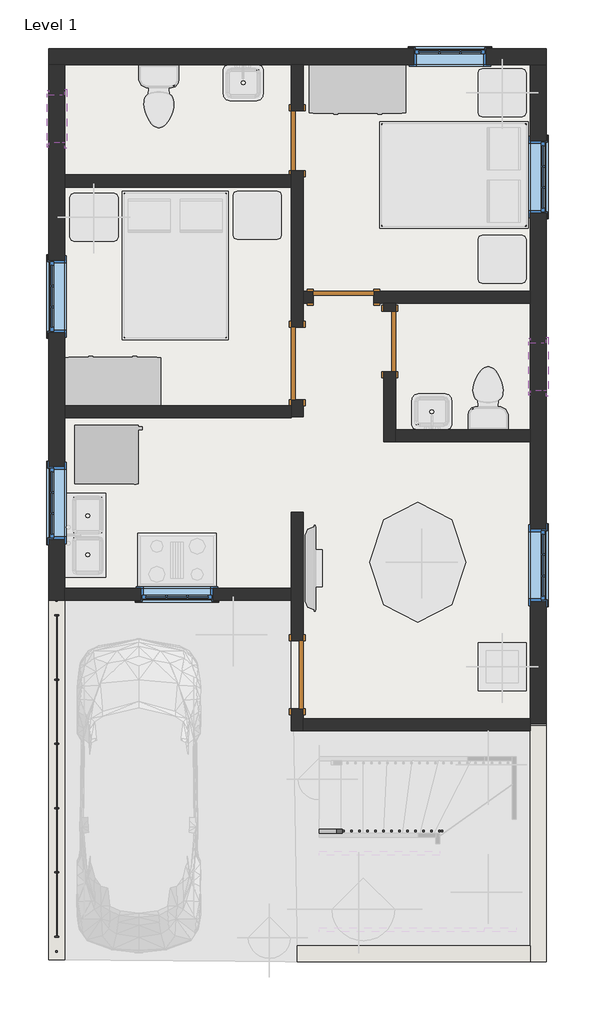
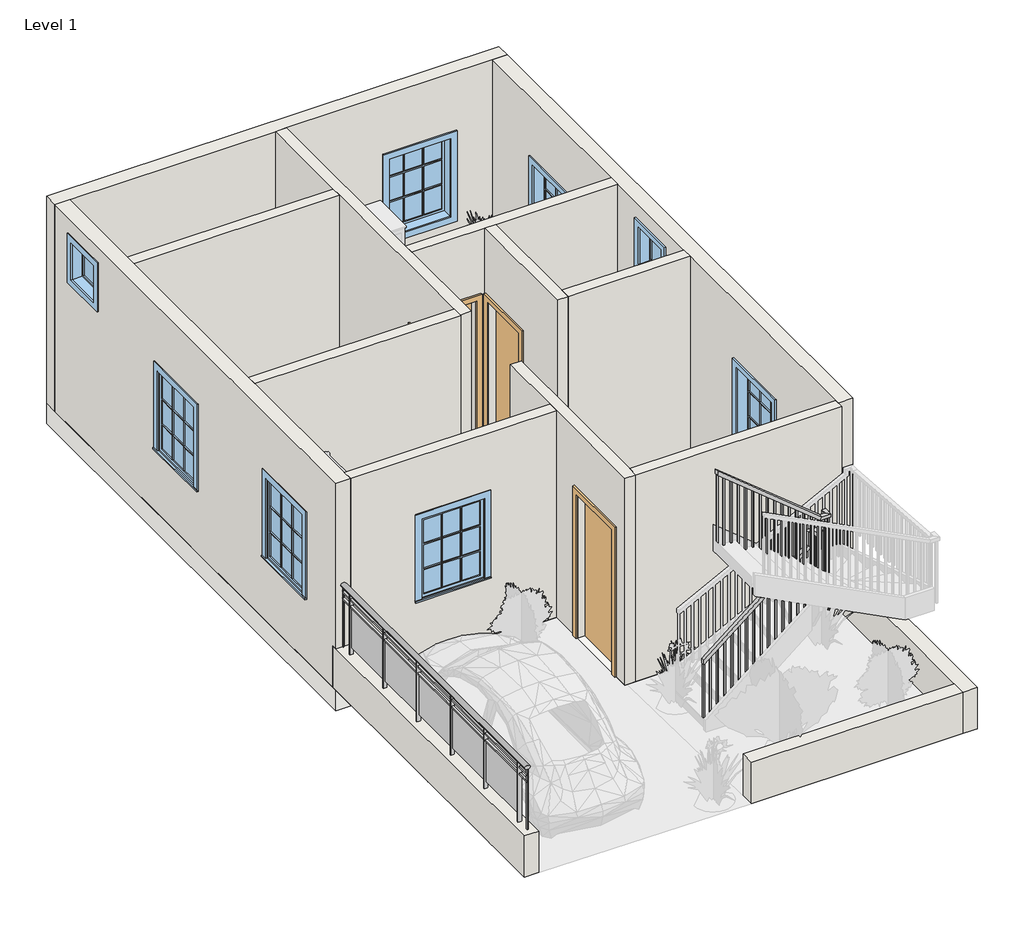
# One storey, part 1 of 2: 15 walls, 8 windows, 5 doors, 2 railings, 1 slab.
"""IFC4 building model written with IfcOpenShell, lengths in millimetres."""

from ifc_helpers import new_model, si_unit, point, frame, origin, origin_with_axes, place, context, project, spatial, polyline, ellipse_curve, trimmed, outline, extrude, faceted_brep, transform, mapped, element, save
from ifc_brep_helpers import plane_surface, extruded_surface, advanced_brep
from components import door_255cab33, door_b6e9fca3, door_686f89d2, window_29c06734, window_5c190c7e, window_e41d21a6

model = new_model("IFC4")

# Units and contexts
model_context = context("Model", 3, world=origin())
ifc_project = project(units=[si_unit("LENGTHUNIT", "METRE", prefix="MILLI")], contexts=[model_context])

# Site, building, storey
site = spatial("IfcSite", under=ifc_project)
building = spatial("IfcBuilding", under=site)
storey = spatial("IfcBuildingStorey", under=building, Name="Level 1", Elevation=0.0)

# Doors
placement = place(None, origin())
door_shape = door_255cab33(model_context)
element("IfcDoor", 1, ObjectType="Single-Flush : 30\" x 80\"", at=placement, inside=storey, context=model_context, shape_type="MappedRepresentation", body=[
    mapped(door_shape, transform((-10291.2586966, 12976.4085318, 0.0), x_axis=(0.0, -1.0, 0.0), y_axis=(1.0, 0.0, 0.0), z_axis=(0.0, 0.0, 1.0))),
])
element("IfcDoor", 2, ObjectType="Single-Flush : 30\" x 80\"", at=placement, inside=storey, context=model_context, shape_type="MappedRepresentation", body=[
    mapped(door_shape, transform((-9707.0586966, 10995.2085318, 0.0), x_axis=(-1.0, 0.0, 0.0), y_axis=(0.0, -1.0, 0.0), z_axis=(0.0, 0.0, 1.0))),
])
element("IfcDoor", 3, ObjectType="Single-Flush : 30\" x 80\"", at=placement, inside=storey, context=model_context, shape_type="MappedRepresentation", body=[
    mapped(door_shape, transform((-9122.8586966, 10436.4085318, 0.0), x_axis=(0.0, 1.0, 0.0), y_axis=(-1.0, 0.0, 0.0), z_axis=(0.0, 0.0, 1.0))),
])
door_2_shape = door_b6e9fca3(model_context)
element("IfcDoor", 4, ObjectType="Single-Flush : 34\" x 84\"", at=placement, inside=storey, context=model_context, shape_type="MappedRepresentation", body=[
    mapped(door_2_shape, transform((-10291.2586966, 6220.0085318, 0.0), x_axis=(0.0, -1.0, 0.0), y_axis=(1.0, 0.0, 0.0), z_axis=(0.0, 0.0, 1.0))),
])
door_3_shape = door_686f89d2(model_context)
element("IfcDoor", 5, ObjectType="Single-Flush : 36\" x 84\"", at=placement, inside=storey, context=model_context, shape_type="MappedRepresentation", body=[
    mapped(door_3_shape, transform((-10291.2586966, 10157.0085318, 0.0), x_axis=(0.0, -1.0, 0.0), y_axis=(1.0, 0.0, 0.0), z_axis=(0.0, 0.0, 1.0))),
])

# Railings
element("IfcRailing", 6, ObjectType="Glass Panel - Bottom Fill", at=placement, inside=storey, context=model_context, shape_type="SolidModel", body=[
    advanced_brep(
    [(-13301.1586966, 7159.8085318, 1524.0), (-13377.3586966, 7159.8085318, 1524.0), (-13301.1586966, 2714.8085318, 1524.0), (-13377.3586966, 2714.8085318, 1524.0)],
    [
        (0, 1, ellipse_curve(frame((-13339.2586966, 7159.8085318, 1524.0), z_axis=(0.0, 1.0, 0.0), x_axis=(-1.0, 0.0, 0.0)), 38.1, 28.575)),
        (1, 0, ellipse_curve(frame((-13339.2586966, 7159.8085318, 1524.0), z_axis=(0.0, 1.0, 0.0), x_axis=(-1.0, 0.0, 0.0)), 38.1, 28.575)),
        (2, 3, ellipse_curve(frame((-13339.2586966, 2714.8085318, 1524.0), z_axis=(0.0, -1.0, 0.0), x_axis=(-1.0, 0.0, 0.0)), 38.1, 28.575)),
        (3, 2, ellipse_curve(frame((-13339.2586966, 2714.8085318, 1524.0), z_axis=(0.0, -1.0, 0.0), x_axis=(-1.0, 0.0, 0.0)), 38.1, 28.575)),
        (0, 2),
        (3, 1),
    ],
    [
        plane_surface(frame((-13339.2586966, 7159.8085318, 1524.0), z_axis=(0.0, 1.0, 0.0), x_axis=(0.0, 0.0, -1.0))),
        plane_surface(frame((-13339.2586966, 2714.8085318, 1524.0), z_axis=(0.0, -1.0, 0.0), x_axis=(0.0, 0.0, -1.0))),
        extruded_surface(trimmed(ellipse_curve(frame((-13339.2586966, 2714.8085318, 1524.0), z_axis=(0.0, 1.0, 0.0), x_axis=(-1.0, 0.0, 0.0)), 38.1, 28.575), [point((-13301.1586966, 2714.8085318, 1524.0))], [point((-13377.3586966, 2714.8085318, 1524.0))], True, "CARTESIAN"), (0.0, 4445.0, 0.0), 4445.0),
        extruded_surface(trimmed(ellipse_curve(frame((-13339.2586966, 2714.8085318, 1524.0), z_axis=(0.0, 1.0, 0.0), x_axis=(-1.0, 0.0, 0.0)), 38.1, 28.575), [point((-13377.3586966, 2714.8085318, 1524.0))], [point((-13301.1586966, 2714.8085318, 1524.0))], True, "CARTESIAN"), (0.0, 4445.0, 0.0), 4445.0),
    ],
    [
        (0, [[1, 2]]),
        (1, [[3, 4]]),
        (2, [[-1, 5, -4, 6]]),
        (3, [[-2, -6, -3, -5]]),
    ],
),
    extrude(outline(polyline([(-13351.9586966, 7159.8085318), (-13326.5586966, 7159.8085318), (-13326.5586966, 2714.8085318), (-13351.9586966, 2714.8085318), (-13351.9586966, 7159.8085318)])), frame((0.0, 0.0, 1409.7), z_axis=(0.0, 0.0, 1.0), x_axis=(1.0, 0.0, 0.0)), (0.0, 0.0, 1.0), 25.4),
    extrude(outline(polyline([(-13351.9586966, 7159.8085318), (-13326.5586966, 7159.8085318), (-13326.5586966, 2714.8085318), (-13351.9586966, 2714.8085318), (-13351.9586966, 7159.8085318)])), frame((0.0, 0.0, 1308.1), z_axis=(0.0, 0.0, 1.0), x_axis=(1.0, 0.0, 0.0)), (0.0, 0.0, 1.0), 25.4),
    extrude(outline(polyline([(-13364.6586966, 2911.6585318), (-13313.8586966, 2911.6585318), (-13313.8586966, 2898.9585318), (-13364.6586966, 2898.9585318), (-13364.6586966, 2911.6585318)])), frame((0.0, 0.0, 609.6), z_axis=(0.0, 0.0, 1.0), x_axis=(1.0, 0.0, 0.0)), (0.0, 0.0, 1.0), 885.6788223),
    extrude(outline(polyline([(-13332.7235395, 3718.1085318), (-13332.7235395, 2905.3085318), (-13339.0735395, 2905.3085318), (-13339.0735395, 3718.1085318), (-13332.7235395, 3718.1085318)])), frame((0.0, 0.0, 711.2), z_axis=(0.0, 0.0, 1.0), x_axis=(1.0, 0.0, 0.0)), (0.0, 0.0, 1.0), 596.9),
    extrude(outline(polyline([(-13364.6586966, 3724.4585318), (-13313.8586966, 3724.4585318), (-13313.8586966, 3711.7585318), (-13364.6586966, 3711.7585318), (-13364.6586966, 3724.4585318)])), frame((0.0, 0.0, 609.6), z_axis=(0.0, 0.0, 1.0), x_axis=(1.0, 0.0, 0.0)), (0.0, 0.0, 1.0), 885.6788223),
    extrude(outline(polyline([(-13332.7235395, 4530.9085318), (-13332.7235395, 3718.1085318), (-13339.0735395, 3718.1085318), (-13339.0735395, 4530.9085318), (-13332.7235395, 4530.9085318)])), frame((0.0, 0.0, 711.2), z_axis=(0.0, 0.0, 1.0), x_axis=(1.0, 0.0, 0.0)), (0.0, 0.0, 1.0), 596.9),
    extrude(outline(polyline([(-13364.6586966, 4537.2585318), (-13313.8586966, 4537.2585318), (-13313.8586966, 4524.5585318), (-13364.6586966, 4524.5585318), (-13364.6586966, 4537.2585318)])), frame((0.0, 0.0, 609.6), z_axis=(0.0, 0.0, 1.0), x_axis=(1.0, 0.0, 0.0)), (0.0, 0.0, 1.0), 885.6788223),
    extrude(outline(polyline([(-13332.7235395, 5343.7085318), (-13332.7235395, 4530.9085318), (-13339.0735395, 4530.9085318), (-13339.0735395, 5343.7085318), (-13332.7235395, 5343.7085318)])), frame((0.0, 0.0, 711.2), z_axis=(0.0, 0.0, 1.0), x_axis=(1.0, 0.0, 0.0)), (0.0, 0.0, 1.0), 596.9),
    extrude(outline(polyline([(-13364.6586966, 5350.0585318), (-13313.8586966, 5350.0585318), (-13313.8586966, 5337.3585318), (-13364.6586966, 5337.3585318), (-13364.6586966, 5350.0585318)])), frame((0.0, 0.0, 609.6), z_axis=(0.0, 0.0, 1.0), x_axis=(1.0, 0.0, 0.0)), (0.0, 0.0, 1.0), 885.6788223),
    extrude(outline(polyline([(-13332.7235395, 6156.5085318), (-13332.7235395, 5343.7085318), (-13339.0735395, 5343.7085318), (-13339.0735395, 6156.5085318), (-13332.7235395, 6156.5085318)])), frame((0.0, 0.0, 711.2), z_axis=(0.0, 0.0, 1.0), x_axis=(1.0, 0.0, 0.0)), (0.0, 0.0, 1.0), 596.9),
    extrude(outline(polyline([(-13364.6586966, 6162.8585318), (-13313.8586966, 6162.8585318), (-13313.8586966, 6150.1585318), (-13364.6586966, 6150.1585318), (-13364.6586966, 6162.8585318)])), frame((0.0, 0.0, 609.6), z_axis=(0.0, 0.0, 1.0), x_axis=(1.0, 0.0, 0.0)), (0.0, 0.0, 1.0), 885.6788223),
    extrude(outline(polyline([(-13332.7235395, 6969.3085318), (-13332.7235395, 6156.5085318), (-13339.0735395, 6156.5085318), (-13339.0735395, 6969.3085318), (-13332.7235395, 6969.3085318)])), frame((0.0, 0.0, 711.2), z_axis=(0.0, 0.0, 1.0), x_axis=(1.0, 0.0, 0.0)), (0.0, 0.0, 1.0), 596.9),
    extrude(outline(polyline([(-13364.6586966, 6975.6585318), (-13313.8586966, 6975.6585318), (-13313.8586966, 6962.9585318), (-13364.6586966, 6962.9585318), (-13364.6586966, 6975.6585318)])), frame((0.0, 0.0, 609.6), z_axis=(0.0, 0.0, 1.0), x_axis=(1.0, 0.0, 0.0)), (0.0, 0.0, 1.0), 885.6788223),
    extrude(outline(polyline([(-13348.7836966, 2727.5085318), (-13329.7336966, 2727.5085318), (-13329.7336966, 2708.4585318), (-13348.7836966, 2708.4585318), (-13348.7836966, 2727.5085318)])), frame((0.0, 0.0, 609.6), z_axis=(0.0, 0.0, 1.0), x_axis=(1.0, 0.0, 0.0)), (0.0, 0.0, 1.0), 885.6788223),
    extrude(outline(polyline([(-13348.7836966, 7166.1585318), (-13329.7336966, 7166.1585318), (-13329.7336966, 7147.1085318), (-13348.7836966, 7147.1085318), (-13348.7836966, 7166.1585318)])), frame((0.0, 0.0, 609.6), z_axis=(0.0, 0.0, 1.0), x_axis=(1.0, 0.0, 0.0)), (0.0, 0.0, 1.0), 885.6788223),
])
element("IfcRailing", 7, ObjectType="Handrail - Rectangular", at=placement, inside=storey, context=model_context, shape_type="SolidModel", body=[
    faceted_brep([(-10015.5903884, 4264.2085318, 1025.2529681), (-10015.5903884, 4264.2085318, 959.7067088), (-10015.5903884, 4213.4085318, 959.7067088), (-10015.5903884, 4213.4085318, 1025.2529681), (-8564.0586966, 4264.2085318, 2208.7848338), (-8513.2586966, 4264.2085318, 2184.659247), (-8513.2586966, 4213.4085318, 2184.659247), (-8564.0586966, 4213.4085318, 2208.7848338), (-8564.0586966, 4264.2085318, 2414.6281882), (-8513.2586966, 4264.2085318, 2363.8281882), (-8513.2586966, 4213.4085318, 2363.8281882), (-8564.0586966, 4213.4085318, 2414.6281882), (-8437.0586966, 4264.2085318, 2414.6281882), (-8437.0586966, 4264.2085318, 2363.8281882), (-8487.8586966, 4213.4085318, 2363.8281882), (-8487.8586966, 4213.4085318, 2414.6281882), (-8437.0586966, 4137.2085318, 2414.6281882), (-8437.0586966, 4108.0871979, 2363.8281882), (-8487.8586966, 4108.0871979, 2363.8281882), (-8487.8586966, 4137.2085318, 2414.6281882), (-8437.0586966, 4010.2085318, 2631.5051451), (-8437.0586966, 3959.4085318, 2617.7256424), (-8487.8586966, 3959.4085318, 2617.7256424), (-8487.8586966, 4010.2085318, 2631.5051451), (-8437.0586966, 4010.2085318, 2837.3484995), (-8437.0586966, 3959.4085318, 2786.5484995), (-8487.8586966, 3959.4085318, 2786.5484995), (-8487.8586966, 4010.2085318, 2837.3484995), (-8437.0586966, 3883.2085318, 2837.3484995), (-8437.0586966, 3883.2085318, 2786.5484995), (-8487.8586966, 3934.0085318, 2786.5484995), (-8487.8586966, 3934.0085318, 2837.3484995), (-8564.0586966, 3883.2085318, 2837.3484995), (-8582.1441096, 3883.2085318, 2786.5484995), (-8582.1441096, 3934.0085318, 2786.5484995), (-8564.0586966, 3934.0085318, 2837.3484995), (-10015.5903884, 3883.2085318, 4020.8803652), (-10015.5903884, 3934.0085318, 4020.8803652), (-10015.5903884, 3934.0085318, 3955.3341059), (-10015.5903884, 3883.2085318, 3955.3341059)], [[[0, 1, 2, 3]], [[1, 0, 4, 5]], [[2, 1, 5, 6]], [[3, 2, 6, 7]], [[0, 3, 7, 4]], [[5, 4, 8, 9]], [[6, 5, 9, 10]], [[7, 6, 10, 11]], [[4, 7, 11, 8]], [[9, 8, 12, 13]], [[10, 9, 13, 14]], [[11, 10, 14, 15]], [[8, 11, 15, 12]], [[13, 12, 16, 17]], [[14, 13, 17, 18]], [[15, 14, 18, 19]], [[12, 15, 19, 16]], [[17, 16, 20, 21]], [[18, 17, 21, 22]], [[19, 18, 22, 23]], [[16, 19, 23, 20]], [[21, 20, 24, 25]], [[22, 21, 25, 26]], [[23, 22, 26, 27]], [[20, 23, 27, 24]], [[25, 24, 28, 29]], [[26, 25, 29, 30]], [[27, 26, 30, 31]], [[24, 27, 31, 28]], [[29, 28, 32, 33]], [[30, 29, 33, 34]], [[31, 30, 34, 35]], [[28, 31, 35, 32]], [[36, 37, 38, 39]], [[33, 32, 36, 39]], [[34, 33, 39, 38]], [[35, 34, 38, 37]], [[32, 35, 37, 36]]]),
    extrude(outline(polyline([(3866.2231262, -9906.3010529), (3881.7558784, -9925.3510529), (2878.6666667, -9925.3510529), (2878.6666667, -9906.3010529), (3866.2231262, -9906.3010529)])), frame((0.0, 3899.0835318, 0.0), z_axis=(0.0, 1.0, 0.0), x_axis=(0.0, 0.0, 1.0)), (0.0, 0.0, 1.0), 19.05),
    extrude(outline(polyline([(3783.3817813, -9804.7010529), (3798.9145334, -9823.7510529), (2878.6666667, -9823.7510529), (2878.6666667, -9804.7010529), (3783.3817813, -9804.7010529)])), frame((0.0, 3899.0835318, 0.0), z_axis=(0.0, 1.0, 0.0), x_axis=(0.0, 0.0, 1.0)), (0.0, 0.0, 1.0), 19.05),
    extrude(outline(polyline([(3700.5404364, -9703.1010529), (3716.0731885, -9722.1510529), (2709.3333333, -9722.1510529), (2709.3333333, -9703.1010529), (3700.5404364, -9703.1010529)])), frame((0.0, 3899.0835318, 0.0), z_axis=(0.0, 1.0, 0.0), x_axis=(0.0, 0.0, 1.0)), (0.0, 0.0, 1.0), 19.05),
    extrude(outline(polyline([(3617.6990914, -9601.5010529), (3633.2318436, -9620.5510529), (2709.3333333, -9620.5510529), (2709.3333333, -9601.5010529), (3617.6990914, -9601.5010529)])), frame((0.0, 3899.0835318, 0.0), z_axis=(0.0, 1.0, 0.0), x_axis=(0.0, 0.0, 1.0)), (0.0, 0.0, 1.0), 19.05),
    extrude(outline(polyline([(3534.8577465, -9499.9010529), (3550.3904987, -9518.9510529), (2709.3333333, -9518.9510529), (2709.3333333, -9499.9010529), (3534.8577465, -9499.9010529)])), frame((0.0, 3899.0835318, 0.0), z_axis=(0.0, 1.0, 0.0), x_axis=(0.0, 0.0, 1.0)), (0.0, 0.0, 1.0), 19.05),
    extrude(outline(polyline([(3452.0164016, -9398.3010529), (3467.5491538, -9417.3510529), (2540.0, -9417.3510529), (2540.0, -9398.3010529), (3452.0164016, -9398.3010529)])), frame((0.0, 3899.0835318, 0.0), z_axis=(0.0, 1.0, 0.0), x_axis=(0.0, 0.0, 1.0)), (0.0, 0.0, 1.0), 19.05),
    extrude(outline(polyline([(3369.1750567, -9296.7010529), (3384.7078088, -9315.7510529), (2540.0, -9315.7510529), (2540.0, -9296.7010529), (3369.1750567, -9296.7010529)])), frame((0.0, 3899.0835318, 0.0), z_axis=(0.0, 1.0, 0.0), x_axis=(0.0, 0.0, 1.0)), (0.0, 0.0, 1.0), 19.05),
    extrude(outline(polyline([(3286.3337117, -9195.1010529), (3301.8664639, -9214.1510529), (2540.0, -9214.1510529), (2540.0, -9195.1010529), (3286.3337117, -9195.1010529)])), frame((0.0, 3899.0835318, 0.0), z_axis=(0.0, 1.0, 0.0), x_axis=(0.0, 0.0, 1.0)), (0.0, 0.0, 1.0), 19.05),
    extrude(outline(polyline([(3203.4923668, -9093.5010529), (3219.025119, -9112.5510529), (2370.6666667, -9112.5510529), (2370.6666667, -9093.5010529), (3203.4923668, -9093.5010529)])), frame((0.0, 3899.0835318, 0.0), z_axis=(0.0, 1.0, 0.0), x_axis=(0.0, 0.0, 1.0)), (0.0, 0.0, 1.0), 19.05),
    extrude(outline(polyline([(3120.6510219, -8991.9010529), (3136.1837741, -9010.9510529), (2370.6666667, -9010.9510529), (2370.6666667, -8991.9010529), (3120.6510219, -8991.9010529)])), frame((0.0, 3899.0835318, 0.0), z_axis=(0.0, 1.0, 0.0), x_axis=(0.0, 0.0, 1.0)), (0.0, 0.0, 1.0), 19.05),
    extrude(outline(polyline([(3037.809677, -8890.3010529), (3053.3424291, -8909.3510529), (2201.3333333, -8909.3510529), (2201.3333333, -8890.3010529), (3037.809677, -8890.3010529)])), frame((0.0, 3899.0835318, 0.0), z_axis=(0.0, 1.0, 0.0), x_axis=(0.0, 0.0, 1.0)), (0.0, 0.0, 1.0), 19.05),
    extrude(outline(polyline([(2954.9683321, -8788.7010529), (2970.5010842, -8807.7510529), (2201.3333333, -8807.7510529), (2201.3333333, -8788.7010529), (2954.9683321, -8788.7010529)])), frame((0.0, 3899.0835318, 0.0), z_axis=(0.0, 1.0, 0.0), x_axis=(0.0, 0.0, 1.0)), (0.0, 0.0, 1.0), 19.05),
    extrude(outline(polyline([(2872.1269871, -8687.1010529), (2887.6597393, -8706.1510529), (2032.0, -8706.1510529), (2032.0, -8687.1010529), (2872.1269871, -8687.1010529)])), frame((0.0, 3899.0835318, 0.0), z_axis=(0.0, 1.0, 0.0), x_axis=(0.0, 0.0, 1.0)), (0.0, 0.0, 1.0), 19.05),
    extrude(outline(polyline([(2789.2856422, -8585.5010529), (2804.8183944, -8604.5510529), (2032.0, -8604.5510529), (2032.0, -8585.5010529), (2789.2856422, -8585.5010529)])), frame((0.0, 3899.0835318, 0.0), z_axis=(0.0, 1.0, 0.0), x_axis=(0.0, 0.0, 1.0)), (0.0, 0.0, 1.0), 19.05),
    extrude(outline(polyline([(4011.297628, 2529.115018), (4030.347628, 2496.5834745), (4030.347628, 1524.0), (4011.297628, 1524.0), (4011.297628, 2529.115018)])), frame((-8471.9836966, 0.0, 0.0), z_axis=(1.0, 0.0, 0.0), x_axis=(0.0, 1.0, 0.0)), (0.0, 0.0, 1.0), 19.05),
    extrude(outline(polyline([(4112.897628, 2355.6134525), (4131.947628, 2323.0819089), (4131.947628, 1524.0), (4112.897628, 1524.0), (4112.897628, 2355.6134525)])), frame((-8471.9836966, 0.0, 0.0), z_axis=(1.0, 0.0, 0.0), x_axis=(0.0, 1.0, 0.0)), (0.0, 0.0, 1.0), 19.05),
    extrude(outline(polyline([(2127.2519138, -8583.6653884), (2111.7191617, -8602.7153884), (1016.0, -8602.7153884), (1016.0, -8583.6653884), (2127.2519138, -8583.6653884)])), frame((0.0, 4229.2835318, 0.0), z_axis=(0.0, 1.0, 0.0), x_axis=(0.0, 0.0, 1.0)), (0.0, 0.0, 1.0), 19.05),
    extrude(outline(polyline([(2044.4105689, -8685.2653884), (2028.8778167, -8704.3153884), (1016.0, -8704.3153884), (1016.0, -8685.2653884), (2044.4105689, -8685.2653884)])), frame((0.0, 4229.2835318, 0.0), z_axis=(0.0, 1.0, 0.0), x_axis=(0.0, 0.0, 1.0)), (0.0, 0.0, 1.0), 19.05),
    extrude(outline(polyline([(1961.569224, -8786.8653884), (1946.0364718, -8805.9153884), (846.6666667, -8805.9153884), (846.6666667, -8786.8653884), (1961.569224, -8786.8653884)])), frame((0.0, 4229.2835318, 0.0), z_axis=(0.0, 1.0, 0.0), x_axis=(0.0, 0.0, 1.0)), (0.0, 0.0, 1.0), 19.05),
    extrude(outline(polyline([(1878.7278791, -8888.4653884), (1863.1951269, -8907.5153884), (846.6666667, -8907.5153884), (846.6666667, -8888.4653884), (1878.7278791, -8888.4653884)])), frame((0.0, 4229.2835318, 0.0), z_axis=(0.0, 1.0, 0.0), x_axis=(0.0, 0.0, 1.0)), (0.0, 0.0, 1.0), 19.05),
    extrude(outline(polyline([(1795.8865341, -8990.0653884), (1780.353782, -9009.1153884), (677.3333333, -9009.1153884), (677.3333333, -8990.0653884), (1795.8865341, -8990.0653884)])), frame((0.0, 4229.2835318, 0.0), z_axis=(0.0, 1.0, 0.0), x_axis=(0.0, 0.0, 1.0)), (0.0, 0.0, 1.0), 19.05),
    extrude(outline(polyline([(1713.0451892, -9091.6653884), (1697.5124371, -9110.7153884), (677.3333333, -9110.7153884), (677.3333333, -9091.6653884), (1713.0451892, -9091.6653884)])), frame((0.0, 4229.2835318, 0.0), z_axis=(0.0, 1.0, 0.0), x_axis=(0.0, 0.0, 1.0)), (0.0, 0.0, 1.0), 19.05),
    extrude(outline(polyline([(1630.2038443, -9193.2653884), (1614.6710921, -9212.3153884), (508.0, -9212.3153884), (508.0, -9193.2653884), (1630.2038443, -9193.2653884)])), frame((0.0, 4229.2835318, 0.0), z_axis=(0.0, 1.0, 0.0), x_axis=(0.0, 0.0, 1.0)), (0.0, 0.0, 1.0), 19.05),
    extrude(outline(polyline([(1547.3624994, -9294.8653884), (1531.8297472, -9313.9153884), (508.0, -9313.9153884), (508.0, -9294.8653884), (1547.3624994, -9294.8653884)])), frame((0.0, 4229.2835318, 0.0), z_axis=(0.0, 1.0, 0.0), x_axis=(0.0, 0.0, 1.0)), (0.0, 0.0, 1.0), 19.05),
    extrude(outline(polyline([(1464.5211545, -9396.4653884), (1448.9884023, -9415.5153884), (508.0, -9415.5153884), (508.0, -9396.4653884), (1464.5211545, -9396.4653884)])), frame((0.0, 4229.2835318, 0.0), z_axis=(0.0, 1.0, 0.0), x_axis=(0.0, 0.0, 1.0)), (0.0, 0.0, 1.0), 19.05),
    extrude(outline(polyline([(1381.6798095, -9498.0653884), (1366.1470574, -9517.1153884), (338.6666667, -9517.1153884), (338.6666667, -9498.0653884), (1381.6798095, -9498.0653884)])), frame((0.0, 4229.2835318, 0.0), z_axis=(0.0, 1.0, 0.0), x_axis=(0.0, 0.0, 1.0)), (0.0, 0.0, 1.0), 19.05),
    extrude(outline(polyline([(1298.8384646, -9599.6653884), (1283.3057124, -9618.7153884), (338.6666667, -9618.7153884), (338.6666667, -9599.6653884), (1298.8384646, -9599.6653884)])), frame((0.0, 4229.2835318, 0.0), z_axis=(0.0, 1.0, 0.0), x_axis=(0.0, 0.0, 1.0)), (0.0, 0.0, 1.0), 19.05),
    extrude(outline(polyline([(1215.9971197, -9701.2653884), (1200.4643675, -9720.3153884), (338.6666667, -9720.3153884), (338.6666667, -9701.2653884), (1215.9971197, -9701.2653884)])), frame((0.0, 4229.2835318, 0.0), z_axis=(0.0, 1.0, 0.0), x_axis=(0.0, 0.0, 1.0)), (0.0, 0.0, 1.0), 19.05),
    extrude(outline(polyline([(1133.1557748, -9802.8653884), (1117.6230226, -9821.9153884), (169.3333333, -9821.9153884), (169.3333333, -9802.8653884), (1133.1557748, -9802.8653884)])), frame((0.0, 4229.2835318, 0.0), z_axis=(0.0, 1.0, 0.0), x_axis=(0.0, 0.0, 1.0)), (0.0, 0.0, 1.0), 19.05),
    extrude(outline(polyline([(1050.3144298, -9904.4653884), (1034.7816777, -9923.5153884), (169.3333333, -9923.5153884), (169.3333333, -9904.4653884), (1050.3144298, -9904.4653884)])), frame((0.0, 4229.2835318, 0.0), z_axis=(0.0, 1.0, 0.0), x_axis=(0.0, 0.0, 1.0)), (0.0, 0.0, 1.0), 19.05),
    extrude(outline(polyline([(-8483.9010529, 3918.1335318), (-8483.9010529, 3899.0835318), (-8502.9510529, 3899.0835318), (-8502.9510529, 3918.1335318), (-8483.9010529, 3918.1335318)])), frame((0.0, 0.0, 1862.6666667), z_axis=(0.0, 0.0, 1.0), x_axis=(1.0, 0.0, 0.0)), (0.0, 0.0, 1.0), 923.8818329),
    extrude(outline(polyline([(-8471.9836966, 3918.1335318), (-8452.9336966, 3918.1335318), (-8452.9336966, 3899.0835318), (-8471.9836966, 3899.0835318), (-8471.9836966, 3918.1335318)])), frame((0.0, 0.0, 1862.6666667), z_axis=(0.0, 0.0, 1.0), x_axis=(1.0, 0.0, 0.0)), (0.0, 0.0, 1.0), 923.8818329),
    extrude(outline(polyline([(-8471.9836966, 3932.9194355), (-8452.9336966, 3932.9194355), (-8452.9336966, 3913.8694355), (-8471.9836966, 3913.8694355), (-8471.9836966, 3932.9194355)])), frame((0.0, 0.0, 1693.3333333), z_axis=(0.0, 0.0, 1.0), x_axis=(1.0, 0.0, 0.0)), (0.0, 0.0, 1.0), 1093.2151662),
    extrude(outline(polyline([(-8471.9836966, 4233.547628), (-8452.9336966, 4233.547628), (-8452.9336966, 4214.497628), (-8471.9836966, 4214.497628), (-8471.9836966, 4233.547628)])), frame((0.0, 0.0, 1354.6666667), z_axis=(0.0, 0.0, 1.0), x_axis=(1.0, 0.0, 0.0)), (0.0, 0.0, 1.0), 1009.1615215),
    extrude(outline(polyline([(-8471.9836966, 4229.2835318), (-8471.9836966, 4248.3335318), (-8452.9336966, 4248.3335318), (-8452.9336966, 4229.2835318), (-8471.9836966, 4229.2835318)])), frame((0.0, 0.0, 1185.3333333), z_axis=(0.0, 0.0, 1.0), x_axis=(1.0, 0.0, 0.0)), (0.0, 0.0, 1.0), 1178.4948549),
    extrude(outline(polyline([(-8502.9510529, 4229.2835318), (-8502.9510529, 4248.3335318), (-8483.9010529, 4248.3335318), (-8483.9010529, 4229.2835318), (-8502.9510529, 4229.2835318)])), frame((0.0, 0.0, 1185.3333333), z_axis=(0.0, 0.0, 1.0), x_axis=(1.0, 0.0, 0.0)), (0.0, 0.0, 1.0), 1178.4948549),
    extrude(outline(polyline([(3939.8013537, -9996.5403884), (3955.3341059, -10015.5903884), (2878.6666667, -10015.5903884), (2878.6666667, -9996.5403884), (3939.8013537, -9996.5403884)])), frame((0.0, 3899.0835318, 0.0), z_axis=(0.0, 1.0, 0.0), x_axis=(0.0, 0.0, 1.0)), (0.0, 0.0, 1.0), 19.05),
    extrude(outline(polyline([(975.239461, -9996.5403884), (959.7067088, -10015.5903884), (169.3333333, -10015.5903884), (169.3333333, -9996.5403884), (975.239461, -9996.5403884)])), frame((0.0, 4229.2835318, 0.0), z_axis=(0.0, 1.0, 0.0), x_axis=(0.0, 0.0, 1.0)), (0.0, 0.0, 1.0), 19.05),
])

# Slab
element("IfcSlab", 8, ObjectType="Generic - 12\"", at=placement, inside=storey, context=model_context, shape_type="SweptSolid", body=[
    extrude(outline(polyline([(-7141.6586966, 14144.8085318), (-7141.6586966, 5508.8085318), (-10367.4586966, 5508.8085318), (-10367.4586966, 7159.8085318), (-13440.8586966, 7159.8085318), (-13440.8586966, 14144.8085318), (-7141.6586966, 14144.8085318)])), frame((0.0, 0.0, -304.8), z_axis=(0.0, 0.0, 1.0), x_axis=(1.0, 0.0, 0.0)), (0.0, 0.0, 1.0), 304.8),
])

# Walls
element("IfcWall", 9, ObjectType="Generic - 2'", at=placement, inside=storey, context=model_context, shape_type="Brep", body=[
    faceted_brep([(-13237.6586966, 2613.2085318, 0.0), (-13237.6586966, 7159.8085318, 0.0), (-13237.6586966, 7236.0085318, 0.0), (-13237.6586966, 7236.0085318, 609.6), (-13237.6586966, 2613.2085318, 609.6), (-13440.8586966, 2613.2085318, 0.0), (-13440.8586966, 2613.2085318, 609.6), (-13440.8586966, 7236.0085318, 609.6), (-13440.8586966, 7236.0085318, 0.0)], [[[0, 1, 2, 3, 4]], [[5, 6, 7, 8]], [[2, 1, 0, 5, 8]], [[3, 2, 8, 7]], [[4, 3, 7, 6]], [[0, 4, 6, 5]]]),
])
element("IfcWall", 10, ObjectType="Generic - 2'", at=placement, inside=storey, context=model_context, shape_type="Brep", body=[
    faceted_brep([(-7344.8586966, 5572.3085318, 0.0), (-7344.8586966, 5508.8085318, 0.0), (-7344.8586966, 2791.0085318, 0.0), (-7344.8586966, 2587.8085318, 0.0), (-7344.8586966, 2587.8085318, 609.6), (-7344.8586966, 2791.0085318, 609.6), (-7344.8586966, 5572.3085318, 609.6), (-7141.6586966, 5572.3085318, 0.0), (-7141.6586966, 5572.3085318, 609.6), (-7141.6586966, 2587.8085318, 609.6), (-7141.6586966, 2587.8085318, 0.0)], [[[0, 1, 2, 3, 4, 5, 6]], [[7, 8, 9, 10]], [[3, 2, 1, 0, 7, 10]], [[6, 5, 4, 9, 8]], [[0, 6, 8, 7]], [[4, 3, 10, 9]]]),
])
element("IfcWall", 11, ObjectType="Generic - 2'", at=placement, inside=storey, context=model_context, shape_type="SweptSolid", body=[
    extrude(outline(polyline([(-10291.2586966, 2791.0085318), (-7344.8586966, 2791.0085318), (-7344.8586966, 2587.8085318), (-10291.2586966, 2587.8085318), (-10291.2586966, 2791.0085318)])), origin_with_axes(), (0.0, 0.0, 1.0), 609.6),
])
element("IfcWall", 12, ObjectType="Generic - 8\"", at=placement, inside=storey, context=model_context, shape_type="Brep", body=[
    faceted_brep([(-13440.8586966, 13941.6085318, 0.0), (-13237.6586966, 13941.6085318, 0.0), (-10367.4586966, 13941.6085318, 0.0), (-10215.0586966, 13941.6085318, 0.0), (-7344.8586966, 13941.6085318, 0.0), (-7141.6586966, 13941.6085318, 0.0), (-7141.6586966, 13941.6085318, 3048.0), (-7344.8586966, 13941.6085318, 3048.0), (-10215.0586966, 13941.6085318, 3048.0), (-10367.4586966, 13941.6085318, 3048.0), (-13237.6586966, 13941.6085318, 3048.0), (-13440.8586966, 13941.6085318, 3048.0), (-7903.6586966, 13941.6085318, 2133.6), (-7903.6586966, 13941.6085318, 914.4), (-8818.0586966, 13941.6085318, 914.4), (-8818.0586966, 13941.6085318, 2133.6), (-13440.8586966, 14144.8085318, 0.0), (-13440.8586966, 14144.8085318, 3048.0), (-7141.6586966, 14144.8085318, 3048.0), (-7141.6586966, 14144.8085318, 0.0), (-7903.6586966, 14144.8085318, 2133.6), (-8818.0586966, 14144.8085318, 2133.6), (-8818.0586966, 14144.8085318, 914.4), (-7903.6586966, 14144.8085318, 914.4)], [[[0, 1, 2, 3, 4, 5, 6, 7, 8, 9, 10, 11], [12, 13, 14, 15]], [[16, 17, 18, 19], [20, 21, 22, 23]], [[5, 4, 3, 2, 1, 0, 16, 19]], [[6, 5, 19, 18]], [[0, 11, 17, 16]], [[13, 12, 20, 23]], [[14, 13, 23, 22]], [[15, 14, 22, 21]], [[12, 15, 21, 20]], [[11, 10, 9, 8, 7, 6, 18, 17]]]),
])
element("IfcWall", 13, ObjectType="Generic - 8\"", at=placement, inside=storey, context=model_context, shape_type="Brep", body=[
    faceted_brep([(-7344.8586966, 13941.6085318, 0.0), (-7344.8586966, 11071.4085318, 0.0), (-7344.8586966, 10919.0085318, 0.0), (-7344.8586966, 9318.8085318, 0.0), (-7344.8586966, 9166.4085318, 0.0), (-7344.8586966, 5597.7085318, 0.0), (-7344.8586966, 5597.7085318, 3048.0), (-7344.8586966, 9166.4085318, 3048.0), (-7344.8586966, 9318.8085318, 3048.0), (-7344.8586966, 10919.0085318, 3048.0), (-7344.8586966, 11071.4085318, 3048.0), (-7344.8586966, 13941.6085318, 3048.0), (-7344.8586966, 7147.1085318, 2133.6), (-7344.8586966, 7147.1085318, 914.4), (-7344.8586966, 8061.5085318, 914.4), (-7344.8586966, 8061.5085318, 2133.6), (-7344.8586966, 12062.0085318, 2133.6), (-7344.8586966, 12062.0085318, 914.4), (-7344.8586966, 12976.4085318, 914.4), (-7344.8586966, 12976.4085318, 2133.6), (-7344.8586966, 9814.1085318, 2768.6), (-7344.8586966, 9814.1085318, 2159.0), (-7344.8586966, 10423.7085318, 2159.0), (-7344.8586966, 10423.7085318, 2768.6), (-7141.6586966, 13941.6085318, 0.0), (-7141.6586966, 13941.6085318, 3048.0), (-7141.6586966, 5597.7085318, 3048.0), (-7141.6586966, 5597.7085318, 0.0), (-7141.6586966, 7147.1085318, 2133.6), (-7141.6586966, 8061.5085318, 2133.6), (-7141.6586966, 8061.5085318, 914.4), (-7141.6586966, 7147.1085318, 914.4), (-7141.6586966, 12062.0085318, 2133.6), (-7141.6586966, 12976.4085318, 2133.6), (-7141.6586966, 12976.4085318, 914.4), (-7141.6586966, 12062.0085318, 914.4), (-7141.6586966, 9814.1085318, 2768.6), (-7141.6586966, 10423.7085318, 2768.6), (-7141.6586966, 10423.7085318, 2159.0), (-7141.6586966, 9814.1085318, 2159.0)], [[[0, 1, 2, 3, 4, 5, 6, 7, 8, 9, 10, 11], [12, 13, 14, 15], [16, 17, 18, 19], [20, 21, 22, 23]], [[24, 25, 26, 27], [28, 29, 30, 31], [32, 33, 34, 35], [36, 37, 38, 39]], [[5, 4, 3, 2, 1, 0, 24, 27]], [[6, 5, 27, 26]], [[0, 11, 25, 24]], [[13, 12, 28, 31]], [[14, 13, 31, 30]], [[15, 14, 30, 29]], [[12, 15, 29, 28]], [[17, 16, 32, 35]], [[18, 17, 35, 34]], [[19, 18, 34, 33]], [[16, 19, 33, 32]], [[21, 20, 36, 39]], [[22, 21, 39, 38]], [[23, 22, 38, 37]], [[20, 23, 37, 36]], [[11, 10, 9, 8, 7, 6, 26, 25]]]),
])
element("IfcWall", 14, ObjectType="Generic - 8\"", at=placement, inside=storey, context=model_context, shape_type="Brep", body=[
    faceted_brep([(-13237.6586966, 7236.0085318, 0.0), (-13237.6586966, 7312.2085318, 0.0), (-13237.6586966, 9471.2085318, 0.0), (-13237.6586966, 9623.6085318, 0.0), (-13237.6586966, 12392.2085318, 0.0), (-13237.6586966, 12544.6085318, 0.0), (-13237.6586966, 13941.6085318, 0.0), (-13237.6586966, 13941.6085318, 3048.0), (-13237.6586966, 12544.6085318, 3048.0), (-13237.6586966, 12392.2085318, 3048.0), (-13237.6586966, 9623.6085318, 3048.0), (-13237.6586966, 9471.2085318, 3048.0), (-13237.6586966, 7312.2085318, 3048.0), (-13237.6586966, 7159.8085318, 3048.0), (-13237.6586966, 7159.8085318, 609.6), (-13237.6586966, 7236.0085318, 609.6), (-13237.6586966, 11465.1085318, 2133.6), (-13237.6586966, 11465.1085318, 914.4), (-13237.6586966, 10550.7085318, 914.4), (-13237.6586966, 10550.7085318, 2133.6), (-13237.6586966, 8848.9085318, 2133.6), (-13237.6586966, 8848.9085318, 914.4), (-13237.6586966, 7934.5085318, 914.4), (-13237.6586966, 7934.5085318, 2133.6), (-13237.6586966, 12951.0085318, 2768.6), (-13237.6586966, 13560.6085318, 2768.6), (-13237.6586966, 13560.6085318, 2159.0), (-13237.6586966, 12951.0085318, 2159.0), (-13440.8586966, 7236.0085318, 0.0), (-13440.8586966, 7236.0085318, 609.6), (-13440.8586966, 7159.8085318, 609.6), (-13440.8586966, 7159.8085318, 3048.0), (-13440.8586966, 13941.6085318, 3048.0), (-13440.8586966, 13941.6085318, 0.0), (-13440.8586966, 11465.1085318, 2133.6), (-13440.8586966, 10550.7085318, 2133.6), (-13440.8586966, 10550.7085318, 914.4), (-13440.8586966, 11465.1085318, 914.4), (-13440.8586966, 8848.9085318, 2133.6), (-13440.8586966, 7934.5085318, 2133.6), (-13440.8586966, 7934.5085318, 914.4), (-13440.8586966, 8848.9085318, 914.4), (-13440.8586966, 12951.0085318, 2768.6), (-13440.8586966, 12951.0085318, 2159.0), (-13440.8586966, 13560.6085318, 2159.0), (-13440.8586966, 13560.6085318, 2768.6)], [[[0, 1, 2, 3, 4, 5, 6, 7, 8, 9, 10, 11, 12, 13, 14, 15], [16, 17, 18, 19], [20, 21, 22, 23], [24, 25, 26, 27]], [[28, 29, 30, 31, 32, 33], [34, 35, 36, 37], [38, 39, 40, 41], [42, 43, 44, 45]], [[6, 5, 4, 3, 2, 1, 0, 28, 33]], [[7, 6, 33, 32]], [[17, 16, 34, 37]], [[18, 17, 37, 36]], [[19, 18, 36, 35]], [[16, 19, 35, 34]], [[21, 20, 38, 41]], [[22, 21, 41, 40]], [[23, 22, 40, 39]], [[20, 23, 39, 38]], [[43, 42, 24, 27]], [[44, 43, 27, 26]], [[45, 44, 26, 25]], [[42, 45, 25, 24]], [[0, 15, 29, 28]], [[14, 30, 29, 15]], [[14, 13, 31, 30]], [[13, 12, 11, 10, 9, 8, 7, 32, 31]]]),
])
element("IfcWall", 15, ObjectType="INNER 6\"", at=placement, inside=storey, context=model_context, shape_type="Brep", body=[
    faceted_brep([(-13237.6586966, 9471.2085318, 0.0), (-10367.4586966, 9471.2085318, 0.0), (-10367.4586966, 9471.2085318, 3048.0), (-13237.6586966, 9471.2085318, 3048.0), (-13237.6586966, 9623.6085318, 0.0), (-13237.6586966, 9623.6085318, 3048.0), (-10367.4586966, 9623.6085318, 3048.0), (-10367.4586966, 9623.6085318, 0.0), (-10367.4586966, 9483.9085318, 0.0), (-10367.4586966, 9483.9085318, 3048.0)], [[[0, 1, 2, 3]], [[4, 5, 6, 7]], [[1, 0, 4, 7, 8]], [[0, 3, 5, 4]], [[2, 1, 8, 7, 6, 9]], [[3, 2, 9, 6, 5]]]),
])
element("IfcWall", 16, ObjectType="INNER 6\"", at=placement, inside=storey, context=model_context, shape_type="SweptSolid", body=[
    extrude(outline(polyline([(-10367.4586966, 12392.2085318), (-13237.6586966, 12392.2085318), (-13237.6586966, 12544.6085318), (-10367.4586966, 12544.6085318), (-10367.4586966, 12392.2085318)])), origin_with_axes(), (0.0, 0.0, 1.0), 3048.0),
])
element("IfcWall", 17, ObjectType="INNER 6\"", at=placement, inside=storey, context=model_context, shape_type="Brep", body=[
    faceted_brep([(-10367.4586966, 7312.2085318, 0.0), (-13237.6586966, 7312.2085318, 0.0), (-13237.6586966, 7312.2085318, 3048.0), (-10367.4586966, 7312.2085318, 3048.0), (-12272.4586966, 7312.2085318, 2133.6), (-12272.4586966, 7312.2085318, 914.4), (-11358.0586966, 7312.2085318, 914.4), (-11358.0586966, 7312.2085318, 2133.6), (-10367.4586966, 7159.8085318, 0.0), (-10367.4586966, 7159.8085318, 3048.0), (-13237.6586966, 7159.8085318, 3048.0), (-13237.6586966, 7159.8085318, 609.6), (-13237.6586966, 7159.8085318, 0.0), (-12272.4586966, 7159.8085318, 2133.6), (-11358.0586966, 7159.8085318, 2133.6), (-11358.0586966, 7159.8085318, 914.4), (-12272.4586966, 7159.8085318, 914.4), (-13237.6586966, 7236.0085318, 0.0)], [[[0, 1, 2, 3], [4, 5, 6, 7]], [[8, 9, 10, 11, 12], [13, 14, 15, 16]], [[1, 0, 8, 12, 17]], [[0, 3, 9, 8]], [[5, 4, 13, 16]], [[6, 5, 16, 15]], [[7, 6, 15, 14]], [[4, 7, 14, 13]], [[1, 17, 12, 11, 10, 2]], [[3, 2, 10, 9]]]),
])
element("IfcWall", 18, ObjectType="INNER 6\"", at=placement, inside=storey, context=model_context, shape_type="Brep", body=[
    faceted_brep([(-10088.0586966, 11071.4085318, 2032.0), (-10088.0586966, 11071.4085318, 0.0), (-10215.0586966, 11071.4085318, 0.0), (-10215.0586966, 11071.4085318, 3048.0), (-7344.8586966, 11071.4085318, 3048.0), (-7344.8586966, 11071.4085318, 0.0), (-9326.0586966, 11071.4085318, 0.0), (-9326.0586966, 11071.4085318, 2032.0), (-10215.0586966, 10919.0085318, 0.0), (-10088.0586966, 10919.0085318, 0.0), (-10088.0586966, 10919.0085318, 2032.0), (-9326.0586966, 10919.0085318, 2032.0), (-9326.0586966, 10919.0085318, 0.0), (-9199.0586966, 10919.0085318, 0.0), (-9046.6586966, 10919.0085318, 0.0), (-7344.8586966, 10919.0085318, 0.0), (-7344.8586966, 10919.0085318, 3048.0), (-9046.6586966, 10919.0085318, 3048.0), (-9199.0586966, 10919.0085318, 3048.0), (-10215.0586966, 10919.0085318, 3048.0)], [[[0, 1, 2, 3, 4, 5, 6, 7]], [[8, 9, 10, 11, 12, 13, 14, 15, 16, 17, 18, 19]], [[6, 5, 15, 14, 13, 12]], [[2, 1, 9, 8]], [[5, 4, 16, 15]], [[3, 2, 8, 19]], [[10, 9, 1, 0]], [[11, 10, 0, 7]], [[12, 11, 7, 6]], [[4, 3, 19, 18, 17, 16]]]),
])
element("IfcWall", 19, ObjectType="INNER 6\"", at=placement, inside=storey, context=model_context, shape_type="Brep", body=[
    faceted_brep([(-9199.0586966, 10919.0085318, 0.0), (-9199.0586966, 10817.4085318, 0.0), (-9199.0586966, 10817.4085318, 2032.0), (-9199.0586966, 10055.4085318, 2032.0), (-9199.0586966, 10055.4085318, 0.0), (-9199.0586966, 9166.4085318, 0.0), (-9199.0586966, 9166.4085318, 3048.0), (-9199.0586966, 10919.0085318, 3048.0), (-9046.6586966, 10817.4085318, 2032.0), (-9046.6586966, 10817.4085318, 0.0), (-9046.6586966, 10919.0085318, 0.0), (-9046.6586966, 10919.0085318, 3048.0), (-9046.6586966, 9318.8085318, 3048.0), (-9046.6586966, 9166.4085318, 3048.0), (-9046.6586966, 9166.4085318, 0.0), (-9046.6586966, 9318.8085318, 0.0), (-9046.6586966, 10055.4085318, 0.0), (-9046.6586966, 10055.4085318, 2032.0)], [[[0, 1, 2, 3, 4, 5, 6, 7]], [[8, 9, 10, 11, 12, 13, 14, 15, 16, 17]], [[10, 9, 1, 0]], [[16, 15, 14, 5, 4]], [[0, 7, 11, 10]], [[6, 5, 14, 13]], [[2, 1, 9, 8]], [[3, 2, 8, 17]], [[4, 3, 17, 16]], [[7, 6, 13, 12, 11]]]),
])
element("IfcWall", 20, ObjectType="INNER 6\"", at=placement, inside=storey, context=model_context, shape_type="SweptSolid", body=[
    extrude(outline(polyline([(-7344.8586966, 9166.4085318), (-9046.6586966, 9166.4085318), (-9046.6586966, 9318.8085318), (-7344.8586966, 9318.8085318), (-7344.8586966, 9166.4085318)])), origin_with_axes(), (0.0, 0.0, 1.0), 3048.0),
])
element("IfcWall", 21, ObjectType="INNER 6\"", at=placement, inside=storey, context=model_context, shape_type="Brep", body=[
    faceted_brep([(-10215.0586966, 5508.8085318, 0.0), (-7344.8586966, 5508.8085318, 0.0), (-7344.8586966, 5508.8085318, 3048.0), (-10215.0586966, 5508.8085318, 3048.0), (-10215.0586966, 5661.2085318, 0.0), (-10215.0586966, 5661.2085318, 3048.0), (-7344.8586966, 5661.2085318, 3048.0), (-7344.8586966, 5661.2085318, 0.0), (-7344.8586966, 5572.3085318, 0.0)], [[[0, 1, 2, 3]], [[4, 5, 6, 7]], [[1, 0, 4, 7, 8]], [[2, 1, 8, 7, 6]], [[0, 3, 5, 4]], [[3, 2, 6, 5]]]),
])
element("IfcWall", 22, ObjectType="INNER 6\"", at=placement, inside=storey, context=model_context, shape_type="Brep", body=[
    faceted_brep([(-10215.0586966, 10614.2085318, 0.0), (-10215.0586966, 10919.0085318, 0.0), (-10215.0586966, 11071.4085318, 0.0), (-10215.0586966, 12595.4085318, 0.0), (-10215.0586966, 12595.4085318, 2032.0), (-10215.0586966, 13357.4085318, 2032.0), (-10215.0586966, 13357.4085318, 0.0), (-10215.0586966, 13941.6085318, 0.0), (-10215.0586966, 13941.6085318, 3048.0), (-10215.0586966, 11071.4085318, 3048.0), (-10215.0586966, 10919.0085318, 3048.0), (-10215.0586966, 9483.9085318, 3048.0), (-10215.0586966, 9483.9085318, 0.0), (-10215.0586966, 9699.8085318, 0.0), (-10215.0586966, 9699.8085318, 2133.6), (-10215.0586966, 10614.2085318, 2133.6), (-10367.4586966, 12595.4085318, 2032.0), (-10367.4586966, 12595.4085318, 0.0), (-10367.4586966, 12544.6085318, 0.0), (-10367.4586966, 12392.2085318, 0.0), (-10367.4586966, 10614.2085318, 0.0), (-10367.4586966, 10614.2085318, 2133.6), (-10367.4586966, 9699.8085318, 2133.6), (-10367.4586966, 9699.8085318, 0.0), (-10367.4586966, 9623.6085318, 0.0), (-10367.4586966, 9483.9085318, 0.0), (-10367.4586966, 9483.9085318, 3048.0), (-10367.4586966, 9623.6085318, 3048.0), (-10367.4586966, 12392.2085318, 3048.0), (-10367.4586966, 12544.6085318, 3048.0), (-10367.4586966, 13941.6085318, 3048.0), (-10367.4586966, 13941.6085318, 0.0), (-10367.4586966, 13357.4085318, 0.0), (-10367.4586966, 13357.4085318, 2032.0)], [[[0, 1, 2, 3, 4, 5, 6, 7, 8, 9, 10, 11, 12, 13, 14, 15]], [[16, 17, 18, 19, 20, 21, 22, 23, 24, 25, 26, 27, 28, 29, 30, 31, 32, 33]], [[32, 31, 7, 6]], [[20, 19, 18, 17, 3, 2, 1, 0]], [[25, 24, 23, 13, 12]], [[12, 11, 26, 25]], [[8, 7, 31, 30]], [[0, 15, 21, 20]], [[15, 14, 22, 21]], [[14, 13, 23, 22]], [[6, 5, 33, 32]], [[5, 4, 16, 33]], [[4, 3, 17, 16]], [[11, 10, 9, 8, 30, 29, 28, 27, 26]]]),
])
element("IfcWall", 23, ObjectType="INNER 6\"", at=placement, inside=storey, context=model_context, shape_type="Brep", body=[
    faceted_brep([(-10215.0586966, 5508.8085318, 0.0), (-10215.0586966, 5661.2085318, 0.0), (-10215.0586966, 5788.2085318, 0.0), (-10215.0586966, 5788.2085318, 2133.6), (-10215.0586966, 6651.8085318, 2133.6), (-10215.0586966, 6651.8085318, 0.0), (-10215.0586966, 8277.4085318, 0.0), (-10215.0586966, 8277.4085318, 3048.0), (-10215.0586966, 5661.2085318, 3048.0), (-10215.0586966, 5508.8085318, 3048.0), (-10367.4586966, 5788.2085318, 2133.6), (-10367.4586966, 5788.2085318, 0.0), (-10367.4586966, 5508.8085318, 0.0), (-10367.4586966, 5508.8085318, 3048.0), (-10367.4586966, 7159.8085318, 3048.0), (-10367.4586966, 7312.2085318, 3048.0), (-10367.4586966, 8277.4085318, 3048.0), (-10367.4586966, 8277.4085318, 0.0), (-10367.4586966, 7312.2085318, 0.0), (-10367.4586966, 7159.8085318, 0.0), (-10367.4586966, 6651.8085318, 0.0), (-10367.4586966, 6651.8085318, 2133.6)], [[[0, 1, 2, 3, 4, 5, 6, 7, 8, 9]], [[10, 11, 12, 13, 14, 15, 16, 17, 18, 19, 20, 21]], [[12, 11, 2, 1, 0]], [[20, 19, 18, 17, 6, 5]], [[7, 6, 17, 16]], [[5, 4, 21, 20]], [[4, 3, 10, 21]], [[3, 2, 11, 10]], [[0, 9, 13, 12]], [[9, 8, 7, 16, 15, 14, 13]]]),
])

# Windows
window_shape = window_29c06734(model_context)
element("IfcWindow", 24, ObjectType="Casement 3x3 with Trim : 36\" x 48\"", at=placement, inside=storey, context=model_context, shape_type="MappedRepresentation", body=[
    mapped(window_shape, transform((-13339.2586966, 11007.9085318, 0.0), x_axis=(0.0, 1.0, 0.0), y_axis=(-1.0, 0.0, 0.0), z_axis=(0.0, 0.0, 1.0))),
])
element("IfcWindow", 25, ObjectType="Casement 3x3 with Trim : 36\" x 48\"", at=placement, inside=storey, context=model_context, shape_type="MappedRepresentation", body=[
    mapped(window_shape, transform((-13339.2586966, 8391.7085318, 0.0), x_axis=(0.0, 1.0, 0.0), y_axis=(-1.0, 0.0, 0.0), z_axis=(0.0, 0.0, 1.0))),
])
element("IfcWindow", 26, ObjectType="Casement 3x3 with Trim : 36\" x 48\"", at=placement, inside=storey, context=model_context, shape_type="MappedRepresentation", body=[
    mapped(window_shape, transform((-7243.2586966, 7604.3085318, 0.0), x_axis=(0.0, -1.0, 0.0), y_axis=(1.0, 0.0, 0.0), z_axis=(0.0, 0.0, 1.0))),
])
element("IfcWindow", 27, ObjectType="Casement 3x3 with Trim : 36\" x 48\"", at=placement, inside=storey, context=model_context, shape_type="MappedRepresentation", body=[
    mapped(window_shape, transform((-7243.2586966, 12519.2085318, 0.0), x_axis=(0.0, -1.0, 0.0), y_axis=(1.0, 0.0, 0.0), z_axis=(0.0, 0.0, 1.0))),
])
element("IfcWindow", 28, ObjectType="Casement 3x3 with Trim : 36\" x 48\"", at=placement, inside=storey, context=model_context, shape_type="MappedRepresentation", body=[
    mapped(window_shape, transform((-8360.8586966, 14043.2085318, 0.0), x_axis=(1.0, 0.0, 0.0), y_axis=(0.0, 1.0, 0.0), z_axis=(0.0, 0.0, 1.0))),
])
window_2_shape = window_5c190c7e(model_context)
element("IfcWindow", 29, ObjectType="Casement 3x3 with Trim : 36\" x 48\"", at=placement, inside=storey, context=model_context, shape_type="MappedRepresentation", body=[
    mapped(window_2_shape, transform((-11815.2586966, 7236.0085318, 0.0), x_axis=(-1.0, 0.0, 0.0), y_axis=(0.0, -1.0, 0.0), z_axis=(0.0, 0.0, 1.0))),
])
window_3_shape = window_e41d21a6(model_context)
element("IfcWindow", 30, ObjectType="Transom with Trim : 24\" x 24\"", at=placement, inside=storey, context=model_context, shape_type="MappedRepresentation", body=[
    mapped(window_3_shape, transform((-13339.2586966, 13217.7085318, 0.0), x_axis=(0.0, -1.0, 0.0), y_axis=(1.0, 0.0, 0.0), z_axis=(0.0, 0.0, 1.0))),
])
element("IfcWindow", 31, ObjectType="Transom with Trim : 24\" x 24\"", at=placement, inside=storey, context=model_context, shape_type="MappedRepresentation", body=[
    mapped(window_3_shape, transform((-7243.2586966, 10080.8085318, 0.0), x_axis=(0.0, -1.0, 0.0), y_axis=(1.0, 0.0, 0.0), z_axis=(0.0, 0.0, 1.0))),
])

save(model, "model.ifc")

# Revit data of these elements
# Type "Single-Flush : 30\" x 80\""
#   Type Mark = "5"
#   Construction Type Id = "MDOOR"
#   Assembly Code = "C1020"
#   Analytic Construction = "Metal"
#   Thickness = 0' - 2"
#   Heat Transfer Coefficient (U) = 0.651978 BTU/(h·ft²·°F)
#   Height = 6' - 8"
#   Trim Projection Ext = 0' - 1"
#   Trim Projection Int = 0' - 1"
#   Trim Width = 0' - 3"
#   Width = 2' - 6"
#   Define Thermal Properties by = 1
#   Door Material = Door - Panel
#   Frame Material = Door - Frame
#   Visual Light Transmittance = 0
#   Solar Heat Gain Coefficient = 0
#   Function = (empty or 0)
#   Wall Closure = (empty or 0)
# Type "Single-Flush : 34\" x 84\""
#   Type Mark = "2"
#   Construction Type Id = "MDOOR"
#   Assembly Code = "C1020"
#   Analytic Construction = "Metal"
#   Thickness = 0' - 2"
#   Heat Transfer Coefficient (U) = 0.651978 BTU/(h·ft²·°F)
#   Height = 7' - 0"
#   Trim Projection Ext = 0' - 1"
#   Trim Projection Int = 0' - 1"
#   Trim Width = 0' - 3"
#   Width = 2' - 10"
#   Define Thermal Properties by = 1
#   Door Material = Door - Panel
#   Frame Material = Door - Frame
#   Visual Light Transmittance = 0
#   Solar Heat Gain Coefficient = 0
#   Function = (empty or 0)
#   Wall Closure = (empty or 0)
# Type "Single-Flush : 36\" x 84\""
#   Type Mark = "1"
#   Construction Type Id = "MDOOR"
#   Assembly Code = "C1020"
#   Analytic Construction = "Metal"
#   Thickness = 0' - 2"
#   Heat Transfer Coefficient (U) = 0.651978 BTU/(h·ft²·°F)
#   Height = 7' - 0"
#   Trim Projection Ext = 0' - 1"
#   Trim Projection Int = 0' - 1"
#   Trim Width = 0' - 3"
#   Width = 3' - 0"
#   Define Thermal Properties by = 1
#   Door Material = Door - Panel
#   Frame Material = Door - Frame
#   Visual Light Transmittance = 0
#   Solar Heat Gain Coefficient = 0
#   Function = (empty or 0)
#   Wall Closure = (empty or 0)
# Type "Glass Panel - Bottom Fill"
#   Assembly Code = "C2010400"
#   built-in parameter 1008612 = 0.0416667 (stored number, unit not read)
#   built-in parameter 1008611 = 0.0416667 (stored number, unit not read)
#   built-in parameter 1008609 = 0.333333 (stored number, unit not read)
#   built-in parameter 1008604 = 0.166667 (stored number, unit not read)
#   built-in parameter 1008603 = 0.166667 (stored number, unit not read)
#   Railing Height = 3' - 0"
#   built-in parameter 1008630 = 2
#   built-in parameter 1008610 = 2
#   built-in parameter 1008618 = Baluster - Square : 3/4"
# Type "Handrail - Rectangular"
#   Assembly Code = "C2010400"
#   built-in parameter 1008612 = 0.0416667 (stored number, unit not read)
#   built-in parameter 1008611 = 0.0416667 (stored number, unit not read)
#   built-in parameter 1008609 = 0.333333 (stored number, unit not read)
#   built-in parameter 1008604 = 0.166667 (stored number, unit not read)
#   built-in parameter 1008603 = 0.166667 (stored number, unit not read)
#   Railing Height = 3' - 0"
#   built-in parameter 1008630 = 2
#   built-in parameter 1008610 = 2
#   built-in parameter 1008618 = Baluster - Square : 3/4"
# Type "Generic - 12\""
#   Assembly Code = "B1010"
#   Function = 0
#   Layers, outside or top first: 1' - 0" no material (function 1)
# Type "Generic - 2'"
#   Assembly Code = "B2010"
#   Layers, outside or top first: 0' - 8" "Birch" (function 1)
# Type "Generic - 8\""
#   Assembly Code = "B2010"
#   Layers, outside or top first: 0' - 8" "Brick, Common" (function 1)
# Type "INNER 6\""
#   Assembly Code = "B2010"
#   Layers, outside or top first: 0' - 6" "Brick, Common" (function 1)
# Type "Casement 3x3 with Trim : 36\" x 48\""
#   Type Mark = "10"
#   Construction Type Id = "GSP4R"
#   Assembly Code = "B2020100"
#   Analytic Construction = "1/8 in Pilkington single glazing"
#   Visual Light Transmittance = 0.9
#   Solar Heat Gain Coefficient = 0.78
#   Heat Transfer Coefficient (U) = 0.6496 BTU/(h·ft²·°F)
#   Height = 4' - 0"
#   Default Sill Height = 3' - 0"
#   Trim Projection - Ext. = 0' - 0 1/2"
#   Trim Projection - Int. = 0' - 0 3/4"
#   Trim Width - Exterior = 0' - 3 1/2"
#   Trim Width - Interior = 0' - 3 1/2"
#   Width = 3' - 0"
#   Window Inset = 0' - 0 3/4"
#   Define Thermal Properties by = 1
#   Glass Pane Material = Glass
#   Sash Material = Sash
#   Trim Exterior Material = Trim
#   Trim Interior Material = Trim
#   Wall Closure = (empty or 0)
# Type "Transom with Trim : 24\" x 24\""
#   Type Mark = "13"
#   Construction Type Id = "GSP4R"
#   Assembly Code = "B2020100"
#   Analytic Construction = "1/8 in Pilkington single glazing"
#   Visual Light Transmittance = 0.9
#   Solar Heat Gain Coefficient = 0.78
#   Heat Transfer Coefficient (U) = 0.6496 BTU/(h·ft²·°F)
#   Height = 2' - 0"
#   Default Sill Height = 7' - 1"
#   Trim Projection - Ext. = 0' - 0 1/2"
#   Trim Projection - Int. = 0' - 0 3/4"
#   Trim Width - Exterior = 0' - 3 1/2"
#   Trim Width - Interior = 0' - 3 1/2"
#   Width = 2' - 0"
#   Window Inset = 0' - 0 3/4"
#   Define Thermal Properties by = 1
#   Glass Pane Material = Glass
#   Sash Material = Sash
#   Trim Exterior Material = Trim
#   Trim Interior Material = Trim
#   Wall Closure = (empty or 0)
# Elements 1, 2, 3 (IfcDoor, "Single-Flush : 30\" x 80\"")
#   Phase Created = New Construction
#   Materials on its faces: "Door - Frame", "Door - Panel"
# Element 4 (IfcDoor, "Single-Flush : 34\" x 84\"")
#   Phase Created = New Construction
#   Materials on its faces: "Door - Frame", "Door - Panel"
# Element 5 (IfcDoor, "Single-Flush : 36\" x 84\"")
#   Phase Created = New Construction
#   Materials on its faces: "Door - Frame", "Door - Panel"
# Element 6 (IfcRailing, "Glass Panel - Bottom Fill")
#   built-in parameter 1008621 = 2 (stored number, unit not read)
#   Phase Created = New Construction
#   Materials on its faces: "Glass"
# Element 7 (IfcRailing, "Handrail - Rectangular")
#   Phase Created = New Construction
# Element 8 (IfcSlab, "Generic - 12\"")
#   Height Offset From Level = 0' - 0"
#   Phase Created = New Construction
#   Materials on its faces: "Default Floor"
# Elements 9, 10, 11 (IfcWall, "Generic - 2'")
#   Top Offset = 0' - 0"
#   Base Offset = 0' - 0"
#   Unconnected Height = 2' - 0"
#   wall height = 2' - 0"
#   Phase Created = New Construction
#   Base Constraint = Level 1
#   Materials on its faces: "Birch"
# Elements 12, 13, 14 (IfcWall, "Generic - 8\"")
#   Top Offset = 0' - 0"
#   Base Offset = 0' - 0"
#   Unconnected Height = 10' - 0"
#   wall height = 10' - 0"
#   Phase Created = New Construction
#   Base Constraint = Level 1
#   Materials on its faces: "Brick, Common"
# Elements 15, 16, 17, 18, 19, 20, 21, 22, 23 (IfcWall, "INNER 6\"")
#   Top Offset = 0' - 0"
#   Base Offset = 0' - 0"
#   Unconnected Height = 10' - 0"
#   wall height = 10' - 0"
#   Phase Created = New Construction
#   Base Constraint = Level 1
#   Materials on its faces: "Brick, Common"
# Element 24 (IfcWindow, "Casement 3x3 with Trim : 36\" x 48\"")
#   Mark = "1"
#   Phase Created = New Construction
#   Materials on its faces: "Sash", "Glass", "Trim"
# Element 25 (IfcWindow, "Casement 3x3 with Trim : 36\" x 48\"")
#   Mark = "2"
#   Phase Created = New Construction
#   Materials on its faces: "Sash", "Glass", "Trim"
# Element 26 (IfcWindow, "Casement 3x3 with Trim : 36\" x 48\"")
#   Mark = "3"
#   Phase Created = New Construction
#   Materials on its faces: "Sash", "Glass", "Trim"
# Element 27 (IfcWindow, "Casement 3x3 with Trim : 36\" x 48\"")
#   Mark = "4"
#   Phase Created = New Construction
#   Materials on its faces: "Sash", "Glass", "Trim"
# Element 28 (IfcWindow, "Casement 3x3 with Trim : 36\" x 48\"")
#   Mark = "5"
#   Phase Created = New Construction
#   Materials on its faces: "Sash", "Glass", "Trim"
# Element 29 (IfcWindow, "Casement 3x3 with Trim : 36\" x 48\"")
#   Mark = "8"
#   Phase Created = New Construction
#   Materials on its faces: "Sash", "Glass", "Trim"
# Element 30 (IfcWindow, "Transom with Trim : 24\" x 24\"")
#   Mark = "6"
#   Phase Created = New Construction
#   Materials on its faces: "Sash", "Trim", "Glass"
# Element 31 (IfcWindow, "Transom with Trim : 24\" x 24\"")
#   Mark = "7"
#   Phase Created = New Construction
#   Materials on its faces: "Sash", "Trim", "Glass"
# Materials
#   "Door - Panel": class "Wood", colour RGB 210 159 95, transparency 0
#   "Door - Frame": colour RGB 118 70 51, transparency 0
#   "Birch": class "Wood", colour RGB 224 178 126, transparency 0, Description = "Betula Alleghaniensis", Cost = 0
#   "Brick, Common": class "Masonry", colour RGB 170 98 104, transparency 0, Description = "Common brick", Cost = 0
#   "Glass": class "Glass", colour RGB 0 128 192, transparency 0.75, Description = "Soda Lime Glass", Cost = 0
#   "Sash": class "Wood", colour RGB 224 178 126, transparency 0
#   "Trim": class "Wood", colour RGB 224 178 126, transparency 0
#   "Default Floor": colour RGB 128 128 128, transparency 0
# Room at (-8687.064, 12292.285) mm, phase "New Construction", upper level "Level 1", upper offset 10' - 0", lower offset 0' - 0"
#   Number = "2"
#   Name = "BEDROOM"
# Room at (-11649.723, 8121.988) mm, phase "New Construction", upper level "Level 1", upper offset 10' - 0", lower offset 0' - 0"
#   Number = "3"
#   Name = "KITCHEN"
# Room at (-8865.193, 7366.608) mm, phase "New Construction", upper level "Level 1", upper offset 10' - 0", lower offset 0' - 0"
#   Number = "6"
# Room at (-12047.381, 13107.841) mm, phase "New Construction", upper level "Level 1", upper offset 10' - 0", lower offset 0' - 0"
#   Number = "1"
# Room at (-11663.167, 11030.13) mm, phase "New Construction", upper level "Level 1", upper offset 10' - 0", lower offset 0' - 0"
#   Number = "4"
#   Name = "BEDROOM"
# Room at (-8246.972, 9937.379) mm, phase "New Construction", upper level "Level 1", upper offset 10' - 0", lower offset 0' - 0"
#   Number = "5"
